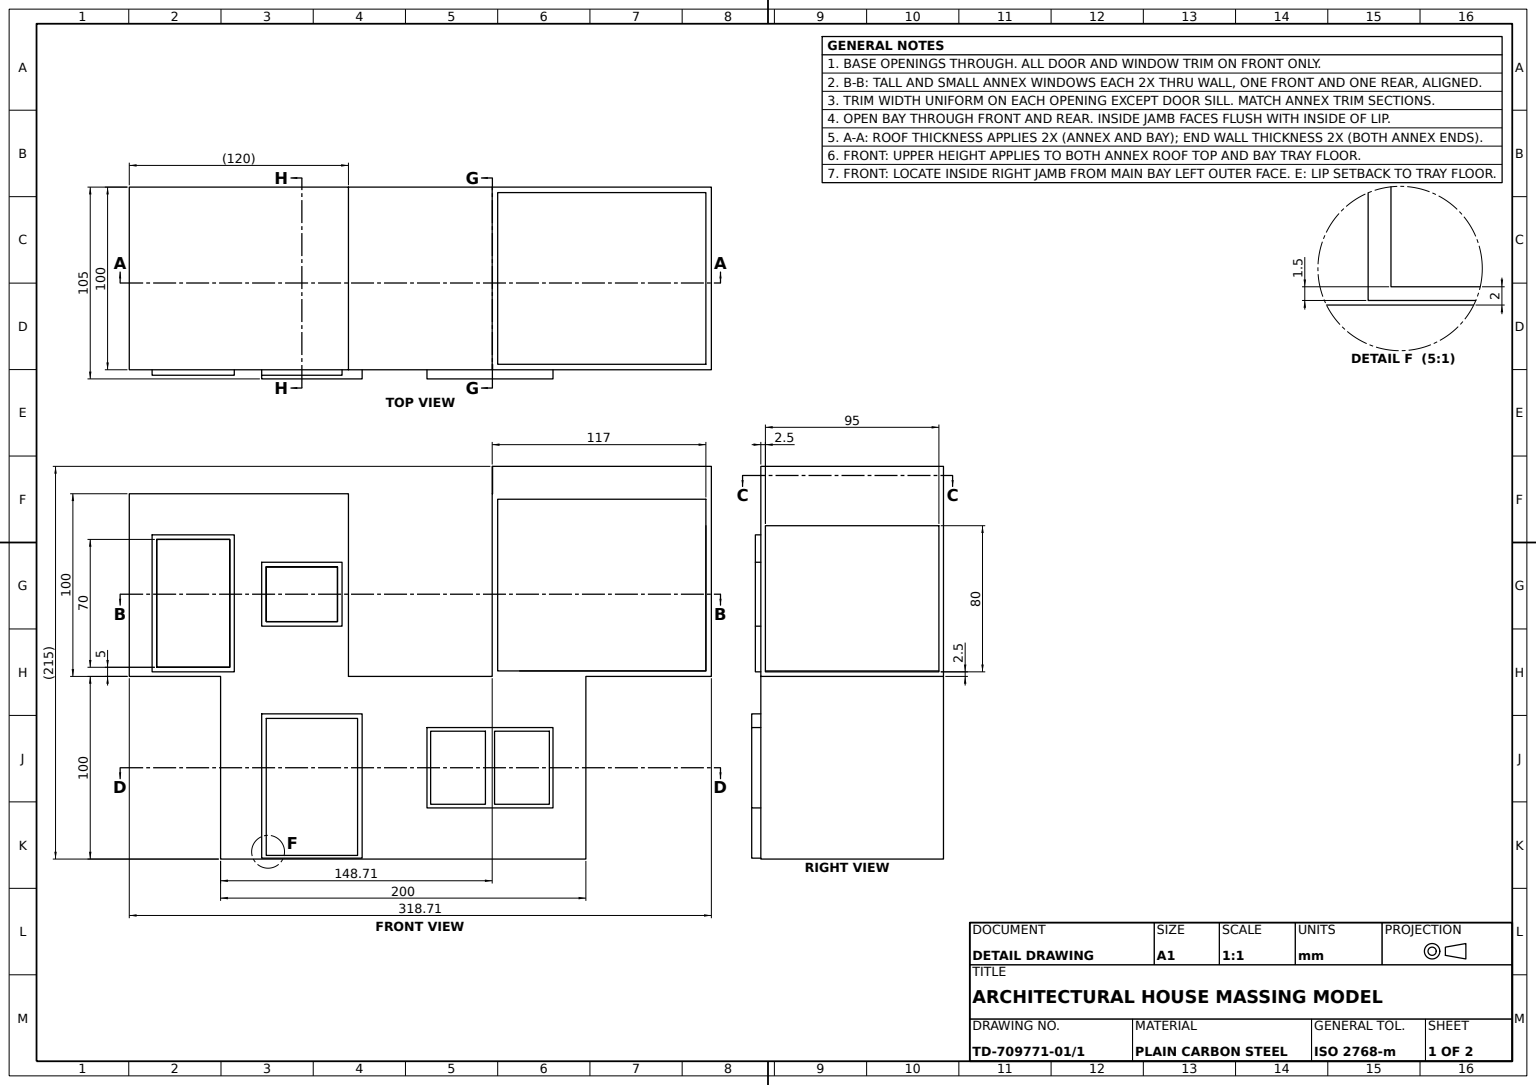
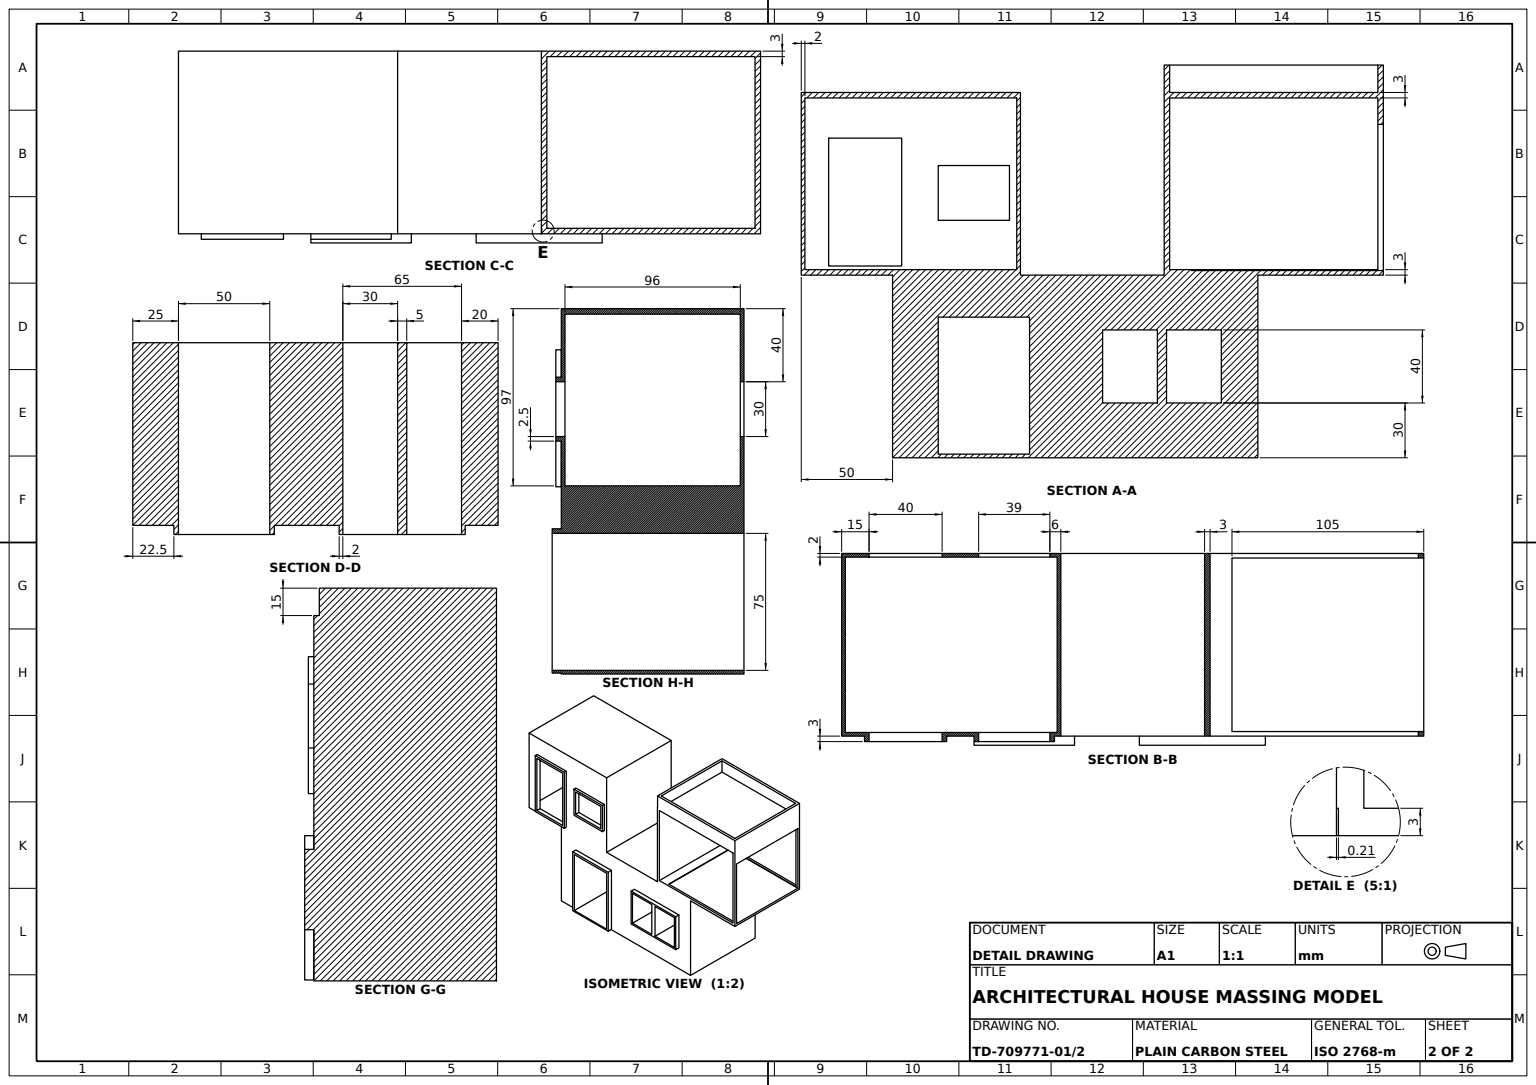
SolidWorks part; units mm, degrees
material "Plain Carbon Steel"
ref_plane "Front Plane" through (0, 0, 0) normal (0, 0, 1) x (1, 0, 0)
ref_plane "Top Plane" through (0, 0, 0) normal (0, 1, 0) x (1, 0, 0)
ref_plane "Right Plane" through (0, 0, 0) normal (1, 0, 0) x (0, 0, -1)
sketch "Base Block Sketch" plane through (0, 0, 0) normal (0, 1, 0) x (1, 0, 0)
  line L1 (0, 0) -> (200, 0)
  line L2 (0, 0) -> (0, 100)
  line L3 (0, 100) -> (200, 100)
  line L4 (200, 0) -> (200, 100)
  dimension "D1" = 200
  dimension "D2" = 100
extrude "Base Block" add sketch "Base Block Sketch" along normal blind 100
sketch "Upper Block Sketch" plane through (0, 100, 0) normal (0, 1, 0) x (1, 0, 0)
  line L0 (200, 100) -> (0, 100) construction
  line L1 (148.7085, 100) -> (268.7085, 100)
  line L2 (148.7085, 100) -> (148.7085, 0)
  line L3 (148.7085, 0) -> (268.7085, 0)
  line L4 (268.7085, 100) -> (268.7085, 0)
  dimension "D1" = 120
  dimension "D2" = 100
  dimension "D3" = 148.7085
extrude "Upper Block" add sketch "Upper Block Sketch" along normal blind 100
sketch "Side Annex Sketch" plane through (0, 100, 0) normal (0, 1, 0) x (1, 0, 0)
  line L0 (148.7085, 100) -> (0, 100) construction
  line L1 (0, 0) -> (70, 0)
  line L3 (0, 100) -> (70, 100)
  line L4 (70, 0) -> (70, 100)
  line L5 (0, 0) -> (-50, 0)
  line L6 (-50, 0) -> (-50, 100)
  line L7 (-50, 100) -> (0, 100)
  dimension "D1" = 70
  dimension "D2" = 50
  dimension "D3" = 70
extrude "Side Annex" add sketch "Side Annex Sketch" along normal blind 100
sketch "Front Door Opening Sketch" plane through (0, 0, 0) normal (0, 0, 1) x (1, 0, 0)
  line L1 (25, 2) -> (75, 2)
  line L2 (25, 2) -> (25, 77)
  line L3 (25, 77) -> (75, 77)
  line L4 (75, 2) -> (75, 77)
  dimension "D1" = 2
  dimension "D2" = 25
  dimension "D3" = 50
  dimension "D4" = 75
extrude "Front Door Opening" cut sketch "Front Door Opening Sketch" against normal blind 100
sketch "Front Window Opening Sketch" plane through (0, 0, 0) normal (0, 0, 1) x (1, 0, 0)
  line L1 (115, 70) -> (180, 70)
  line L2 (115, 70) -> (115, 30)
  line L3 (115, 30) -> (180, 30)
  line L4 (180, 70) -> (180, 30)
  dimension "D1" = 20
  dimension "D2" = 65
  dimension "D3" = 40
  dimension "D4" = 30
extrude "Front Window Opening" cut sketch "Front Window Opening Sketch" against normal blind 100
sketch "Front Window Mullion Sketch" plane through (0, 0, 0) normal (0, 0, 1) x (1, 0, 0)
  line L0 (180, 70) -> (115, 70) construction
  line L1 (145, 70) -> (150, 70)
  line L2 (145, 70) -> (145, 30)
  line L3 (145, 30) -> (150, 30)
  line L4 (150, 70) -> (150, 30)
  line L5 (115, 30) -> (180, 30) construction
  dimension "D1" = 5
  dimension "D2" = 30
extrude "Front Window Mullion" add sketch "Front Window Mullion Sketch" against normal blind 100
sketch "Front Window Frame Sketch" plane through (0, 0, 0) normal (0, 0, 1) x (1, 0, 0)
  line L0 (115, 30) -> (145, 30) construction
  line L1 (113, 72) -> (182, 72)
  line L2 (113, 72) -> (113, 28)
  line L3 (113, 28) -> (182, 28)
  line L4 (182, 72) -> (182, 28)
  line L5 (145, 70) -> (115, 70) construction
  line L6 (180, 30) -> (180, 70) construction
  line L8 (115, 30) -> (145, 30)
  line L9 (115, 30) -> (115, 70)
  line L10 (115, 70) -> (145, 70)
  line L11 (145, 30) -> (145, 70)
  line L12 (150, 30) -> (180, 30)
  line L13 (150, 30) -> (150, 70)
  line L14 (150, 70) -> (180, 70)
  line L15 (180, 30) -> (180, 70)
  dimension "D1" = 2
  dimension "D2" = 2
  dimension "D3" = 2
  dimension "D4" = 2
extrude "Front Window Frame" add sketch "Front Window Frame Sketch" along normal blind 5
sketch "Front Door Frame Sketch" plane through (0, 0, 0) normal (0, 0, 1) x (1, 0, 0)
  line L1 (22.5, 0.5) -> (77.5, 0.5)
  line L2 (22.5, 0.5) -> (22.5, 79.5)
  line L3 (22.5, 79.5) -> (77.5, 79.5)
  line L4 (77.5, 0.5) -> (77.5, 79.5)
  line L5 (75, 2) -> (75, 77) construction
  line L7 (25, 2) -> (75, 2) construction
  line L8 (75, 77) -> (25, 77) construction
  line L10 (25, 2) -> (75, 2)
  line L11 (25, 2) -> (25, 77)
  line L12 (25, 77) -> (75, 77)
  line L13 (75, 2) -> (75, 77)
  dimension "D1" = 22.5
  dimension "D2" = 2.5
  dimension "D3" = 1.5
  dimension "D4" = 2.5
extrude "Front Door Frame" add sketch "Front Door Frame Sketch" along normal blind 5
sketch "Upper Block Hollow Sketch" plane through (0, 0, 0) normal (0, 0, 1) x (1, 0, 0)
  line L0 (268.7085, 200) -> (268.7085, 100) construction
  line L1 (265.7085, 103) -> (151.7085, 103)
  line L2 (265.7085, 103) -> (265.7085, 197)
  line L3 (265.7085, 197) -> (151.7085, 197)
  line L4 (151.7085, 103) -> (151.7085, 197)
  line L5 (200, 100) -> (268.7085, 100) construction
  line L6 (148.7085, 200) -> (148.7085, 100) construction
  line L7 (148.7085, 200) -> (268.7085, 200) construction
  dimension "D1" = 3
  dimension "D2" = 3
  dimension "D3" = 3
  dimension "D4" = 3
extrude "Upper Block Hollow" cut sketch "Upper Block Hollow Sketch" against normal blind 125
sketch "Upper Interior Cut Sketch" plane through (268.7085, 0, 0) normal (1, 0, 0) x (0, 0, -1)
  line L0 (100, 200) -> (100, 100) construction
  line L1 (97.5, 102.5) -> (2.5, 102.5)
  line L2 (97.5, 102.5) -> (97.5, 182.5)
  line L3 (97.5, 182.5) -> (2.5, 182.5)
  line L4 (2.5, 102.5) -> (2.5, 182.5)
  line L5 (0, 200) -> (0, 100) construction
  line L6 (0, 100) -> (100, 100) construction
  dimension "D1" = 2.5
  dimension "D2" = 2.5
  dimension "D3" = 2.5
  dimension "D4" = 80
extrude "Upper Interior Cut" cut sketch "Upper Interior Cut Sketch" against normal blind 105
sketch "Upper Frame Member 1 Sketch" plane through (268.7085, 0, 0) normal (1, 0, 0) x (0, 0, -1)
  line L1 (0, 200) -> (100, 200)
  line L2 (0, 200) -> (0, 215)
  line L3 (0, 215) -> (100, 215)
  line L4 (100, 200) -> (100, 215)
  dimension "D1" = 15
  dimension "D2" = 100
extrude "Upper Frame Member 1" add sketch "Upper Frame Member 1 Sketch" against normal blind 3
sketch "Upper Frame Member 2 Sketch" plane through (0, 0, 0) normal (0, 0, 1) x (1, 0, 0)
  line L1 (265.7085, 200) -> (148.9209, 200)
  line L2 (265.7085, 200) -> (265.7085, 215)
  line L3 (265.7085, 215) -> (148.9209, 215)
  line L4 (148.9209, 200) -> (148.9209, 215)
  dimension "D1" = 116.7875
  dimension "D2" = 15
extrude "Upper Frame Member 2" add sketch "Upper Frame Member 2 Sketch" against normal blind 3
sketch "Upper Frame Member 3 Sketch" plane through (148.7085, 0, 0) normal (-1, 0, 0) x (0, 0, 1)
  line L1 (-3, 200) -> (-100, 200)
  line L2 (-3, 200) -> (-3, 215)
  line L3 (-3, 215) -> (-100, 215)
  line L4 (-100, 200) -> (-100, 215)
extrude "Upper Frame Member 3" add sketch "Upper Frame Member 3 Sketch" against normal blind 3
sketch "Upper Frame Member 4 Sketch" plane through (0, 0, -100) normal (0, 0, -1) x (-1, 0, 0)
  line L1 (-265.7085, 200) -> (-151.7085, 200)
  line L2 (-265.7085, 200) -> (-265.7085, 215)
  line L3 (-265.7085, 215) -> (-151.7085, 215)
  line L4 (-151.7085, 200) -> (-151.7085, 215)
extrude "Upper Frame Member 4" add sketch "Upper Frame Member 4 Sketch" against normal blind 3
sketch "Annex Door Opening Sketch" plane through (0, 0, 0) normal (0, 0, 1) x (1, 0, 0)
  line L1 (-35, 105) -> (5, 105)
  line L2 (-35, 105) -> (-35, 175)
  line L3 (-35, 175) -> (5, 175)
  line L4 (5, 105) -> (5, 175)
  dimension "D1" = 5
  dimension "D2" = 15
  dimension "D3" = 40
  dimension "D4" = 70
extrude "Annex Door Opening" cut sketch "Annex Door Opening Sketch" against normal blind 153
sketch "Annex Window Opening Sketch" plane through (0, 0, 0) normal (0, 0, 1) x (1, 0, 0)
  line L0 (70, 200) -> (70, 100) construction
  line L1 (25, 130) -> (64, 130)
  line L2 (25, 130) -> (25, 160)
  line L3 (25, 160) -> (64, 160)
  line L4 (64, 130) -> (64, 160)
  dimension "D1" = 6
  dimension "D2" = 20
  dimension "D3" = 30
  dimension "D4" = 40
extrude "Annex Window Opening" cut sketch "Annex Window Opening Sketch" against normal blind 153
sketch "Annex Door Frame Sketch" plane through (0, 0, 0) normal (0, 0, 1) x (1, 0, 0)
  line L0 (-35, 175) -> (-35, 105) construction
  line L1 (-37.5, 102.5) -> (7.5, 102.5)
  line L2 (-37.5, 102.5) -> (-37.5, 177.5)
  line L3 (-37.5, 177.5) -> (7.5, 177.5)
  line L4 (7.5, 102.5) -> (7.5, 177.5)
  line L5 (5, 105) -> (5, 175) construction
  line L6 (5, 175) -> (-35, 175) construction
  line L7 (-35, 105) -> (5, 105) construction
  line L9 (-35, 105) -> (5, 105)
  line L10 (-35, 105) -> (-35, 175)
  line L11 (-35, 175) -> (5, 175)
  line L12 (5, 105) -> (5, 175)
  dimension "D1" = 2.5
  dimension "D2" = 2.5
  dimension "D3" = 2.5
  dimension "D4" = 2.5
extrude "Annex Door Frame" add sketch "Annex Door Frame Sketch" along normal blind 3
sketch "Annex Window Frame Sketch" plane through (0, 0, 0) normal (0, 0, 1) x (1, 0, 0)
  line L0 (64, 130) -> (64, 160) construction
  line L1 (22.5, 127.5) -> (66.5, 127.5)
  line L2 (22.5, 127.5) -> (22.5, 162.5)
  line L3 (22.5, 162.5) -> (66.5, 162.5)
  line L4 (66.5, 127.5) -> (66.5, 162.5)
  line L5 (64, 160) -> (25, 160) construction
  line L6 (25, 160) -> (25, 130) construction
  line L7 (25, 130) -> (64, 130) construction
  line L9 (25, 130) -> (64, 130)
  line L10 (25, 130) -> (25, 160)
  line L11 (25, 160) -> (64, 160)
  line L12 (64, 130) -> (64, 160)
  dimension "D1" = 2.5
  dimension "D2" = 2.5
  dimension "D3" = 2.5
  dimension "D4" = 2.5
extrude "Annex Window Frame" add sketch "Annex Window Frame Sketch" along normal blind 3
sketch "Annex Hollow Sketch" plane through (0, 200, 0) normal (0, 1, 0) x (1, 0, 0)
  line L0 (-50, 0) -> (70, 0) construction
  line L1 (-48, 2) -> (68, 2)
  line L2 (-48, 2) -> (-48, 98)
  line L3 (-48, 98) -> (68, 98)
  line L4 (68, 2) -> (68, 98)
  line L5 (70, 0) -> (70, 100) construction
  line L6 (70, 100) -> (-50, 100) construction
  line L7 (-50, 100) -> (-50, 0) construction
  dimension "D1" = 2
  dimension "D2" = 2
  dimension "D3" = 2
  dimension "D4" = 2
extrude "Annex Hollow" cut sketch "Annex Hollow Sketch" against normal blind 97
sketch "Annex Rim Sketch" plane through (0, 200, 0) normal (0, 1, 0) x (1, 0, 0)
  line L1 (-50, 0) -> (70, 0)
  line L2 (-50, 0) -> (-50, 100)
  line L3 (-50, 100) -> (70, 100)
  line L4 (70, 0) -> (70, 100)
extrude "Annex Rim" add sketch "Annex Rim Sketch" against normal blind 3
